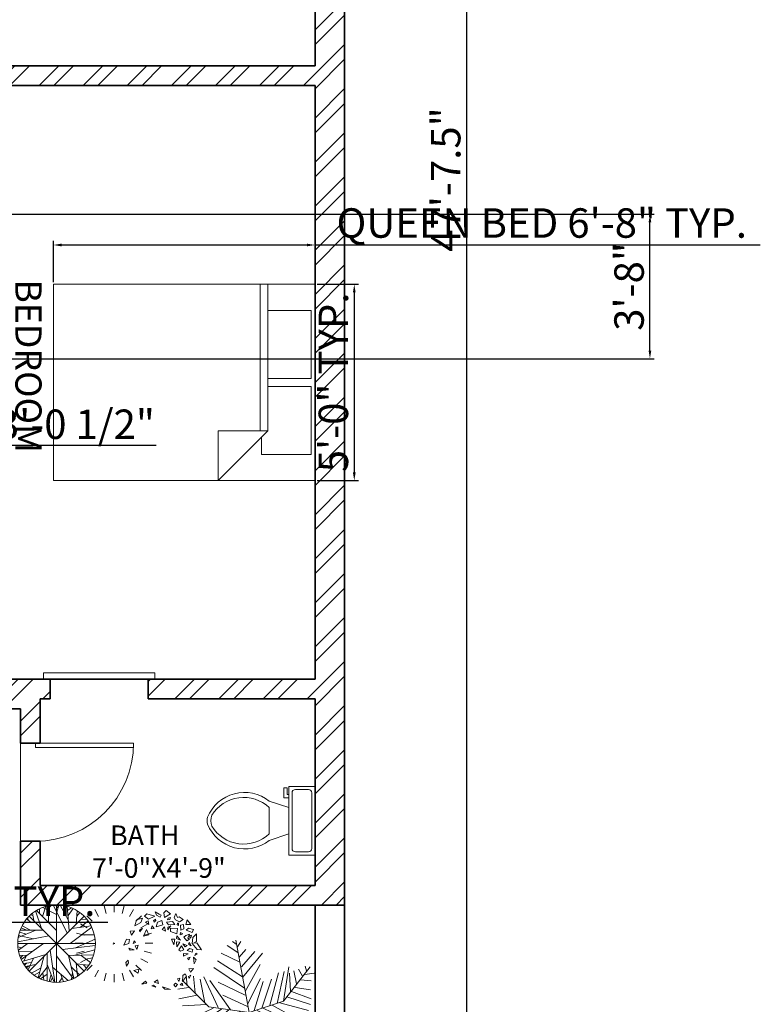
# Model space of a CAD drawing. Units: inches. Extents: x 744 to 1448, y 5126 to 6077.
# Tile 4 of 10: x 1221 to 1448, y 5284 to 5585. Entities that reach past the tile are written whole.
import ezdxf

# ---------------------------------------------------------------- set-up
doc = ezdxf.new("R2010")
doc.units = ezdxf.units.IN
for name, color, linetype, lineweight in [('A-ANNO-DIMS', 2, 'Continuous', 18), ('A-AREA-IDEN', 7, 'Continuous', 18), ('A-DOOR', 4, 'Continuous', 18), ('A-FLOR-FIXT', 9, 'Continuous', 18), ('A-FURN', 8, 'Continuous', 18), ('A-WALL', 7, 'Continuous', 35), ('A-WALL-PATT', 252, 'Continuous', 13), ('L-PLNT', 3, 'Continuous', 13)]:
    doc.layers.add(name, color=color, linetype=linetype, lineweight=lineweight)
doc.styles.get("Standard").update_dxf_attribs({"font": 'arial.ttf'})
doc.dimstyles.new('ISO-25', dxfattribs={"dimtxt": 9, "dimasz": 2.5, "dimexe": 1.25, "dimexo": 0.625, "dimtad": 1, "dimlunit": 3, "dimtxsty": 'Standard', "dimcen": 2.5, "dimadec": 0, "dimazin": 0, "dimtfac": 1, "dimtmove": 0, "dimatfit": 3, "dimfxl": 1, "dimarcsym": 0})

# ---------------------------------------------------------------- blocks, each defined once
blk = doc.blocks.new('*U3')
for p, q in [((-40, 0), (-40, 6)), ((0, 0), (0, 6))]:
    blk.add_line(p, q)
blk.add_lwpolyline([(0, 0), (0, -40), (-1.75, -40), (-1.75, 0)], close=True)
blk.add_arc((0, 0), 40, 180, 270)
blk = doc.blocks.new('*U8')
for p, q in [((9.5, -6), (9.5, -2)), ((-10, -8.5), (-8, -8.5)), ((-10, -9.5), (-10, -8.5)), ((-8, -8.5), (-8, -8)), ((-7, -8), (-7, -9.5)), ((-4, -8), (-6, -14)), ((4, -8), (6, -14)), ((-7, -9.5), (-10, -9.5)), ((4, -14), (-4, -14))]:
    blk.add_line(p, q)
blk.add_lwpolyline([(10.5, -8), (10.5, 0), (-10.5, 0), (-10.5, -8)], close=True)
for points in [[(-9.5, -2), (-9.5, -6)], [(8.5, -1), (-8.5, -1)], [(-8.5, -7), (8.5, -7)]]:
    blk.add_lwpolyline(points)
for centre, radius, start, end in [((-8.62, -1.88), 0.884, 81.8699, 188.1301), ((8.62, -1.88), 0.884, 351.8699, 98.1301), ((-8.62, -6.12), 0.884, 171.8699, 278.1301), ((8.62, -6.12), 0.884, 261.8699, 8.1301), ((3.52, -21.58), 12.17, 141.4691, 247.9714), ((4.2, -21.82), 11.33, 136.3677, 238.9468), ((-3.52, -21.58), 12.17, 292.0284, 38.5307), ((-4.2, -21.82), 11.33, 301.053, 43.6321), ((0, -27.88), 4, 245.7318, 294.2682), ((0, -29), 4, 254.8605, 285.1395)]:
    blk.add_arc(centre, radius, start, end)
blk = doc.blocks.new('*U10')
for p, q in [((-10.186, 53.64), (-13.084, 55.962)), ((0, 0), (-10.5, 57)), ((-9.099, 51.782), (-6.563, 55.962)), ((-7.288, 39.707), (-21.778, 46.673)), ((-8.737, 47.138), (-17.069, 52.711)), ((-7.65, 43.423), (-2.578, 49.46)), ((-5.839, 35.992), (4.667, 48.067)), ((-5.114, 27.632), (10.463, 46.673)), ((-5.114, 28.097), (-24.676, 40.636)), ((-3.665, 19.273), (-27.574, 35.527)), ((-2.941, 16.486), (8.652, 37.85)), ((16.259, 5.805), (23.142, 31.348)), ((22.055, 7.198), (27.489, 32.277)), ((27, 9), (48, 36)), ((27.127, 9.056), (31.112, 35.992)), ((35.096, 32.741), (37.27, 22.524)), ((38.719, 34.134), (41.979, 28.561)), ((44.153, 36.456), (45.239, 32.741)), ((-31.5, 4.5), (-52.5, 25.5)), ((-48.585, 21.131), (-49.309, 29.026)), ((-43.513, 28.561), (-42.427, 15.558)), ((-38.442, 26.239), (-34.819, 7.663)), ((-35.544, 28.097), (-24.314, 3.947)), ((-14.533, 2.09), (-30.834, 25.31)), ((-24.314, 23.917), (-2.941, 13.7)), ((-1.129, 6.734), (9.014, 26.704)), ((3.942, 1.625), (11.187, 24.381)), ((10.101, 3.483), (17.708, 26.239)), ((31.836, 30.883), (32.561, 16.486)), ((40.53, 25.775), (48.862, 24.846)), ((43.791, 29.954), (51.036, 30.883)), ((-47.498, 19.737), (-55.83, 18.344)), ((33.285, 16.486), (48.862, 10.913)), ((36.183, 19.737), (48.137, 17.88)), ((-40.615, 13.7), (-55.105, 10.913)), ((-20.691, 13.7), (-1.129, 4.876)), ((0, 0), (27, 9)), ((29.662, 12.307), (48.137, 6.269)), ((-33.37, 6.269), (-52.207, 5.34)), ((-28.299, 3.483), (-47.86, -5.805)), ((-21.416, 3.018), (-38.079, -8.128)), ((0, 0), (-31.5, 4.5)), ((-15.982, 2.09), (-30.11, -9.521)), ((0, 0), (-22.5, -19.5)), ((-6.563, 1.161), (-21.416, -8.128)), ((0, 0), (18, -22.5)), ((6.478, 1.625), (26.04, -8.592)), ((11.187, 3.483), (30.749, -5.805)), ((18.07, 5.805), (35.096, -3.483)), ((24.229, 7.663), (46.688, 1.625)), ((-6.563, -5.805), (-19.967, -9.985)), ((-4.752, -3.483), (-3.665, -14.629)), ((2.493, -3.019), (-1.491, -20.202)), ((1.769, -2.555), (24.229, -9.521)), ((5.029, -6.27), (2.131, -25.775)), ((-17.431, -15.094), (-42.789, -18.809)), ((-15.257, -12.772), (-30.11, -12.772)), ((-17.069, -15.094), (-12.721, -40.172)), ((-13.446, -11.378), (-8.737, -32.741)), ((-9.461, -8.592), (-6.201, -23.453)), ((9.014, -11.378), (3.58, -35.992)), ((7.565, -9.056), (32.198, -14.629)), ((12.274, -15.094), (36.907, -18.809)), ((-24.314, -21.596), (-42.427, -22.06)), ((-22.5, -19.5), (-37.5, -45)), ((-20.691, -18.345), (-17.793, -44.352)), ((14.085, -16.951), (6.478, -40.172)), ((18.07, -22.524), (8.289, -45.745)), ((16.259, -19.738), (36.183, -22.989)), ((18, -22.5), (27, -52.5)), ((18.433, -22.524), (40.53, -29.026)), ((-28.299, -29.026), (-42.789, -31.348)), ((-26.849, -26.24), (-40.253, -25.775)), ((-29.023, -30.884), (-27.936, -43.887)), ((-25.038, -23.918), (-22.865, -45.281)), ((20.244, -30.419), (15.897, -44.816)), ((19.157, -25.311), (38.719, -33.206)), ((-30.834, -34.135), (-42.427, -35.528)), ((-32.646, -36.921), (-31.921, -44.352)), ((22.78, -37.85), (19.519, -48.532)), ((21.331, -32.741), (39.081, -40.636)), ((22.78, -38.314), (34.372, -44.816)), ((-34.457, -39.708), (-40.978, -42.494)), ((24.591, -45.745), (23.142, -50.854)), ((24.591, -43.423), (30.749, -47.603)), ((26.764, -49.925), (28.213, -50.854))]:
    blk.add_line(p, q)
blk = doc.blocks.new('*U11')
for points in [[(1.24, 12), (0.56, 11.31), (0.76, 10.01), (2.52, 11.05)], [(-5.78, 9.75), (-7.54, 9.23), (-8.01, 7.5), (-6.26, 8.45)], [(-4.43, 11.05), (-5.18, 10.36), (-3.96, 9.49), (-2.07, 10.36)], [(-4.84, 8.63), (-3.83, 7.85), (-4.03, 8.97)], [(-1.94, 9.49), (-2.48, 8.97), (-2.27, 8.54), (-1.8, 9.06)], [(-2, 11.66), (-1.6, 10.62), (-0.52, 10.1), (-0.18, 10.62), (-0.79, 10.96)], [(0.02, 9.06), (-1.33, 8.54), (-1.73, 7.16), (0.29, 7.76)], [(1.37, 8.54), (3.13, 8.8), (3.8, 7.85), (1.91, 7.76)], [(2.59, 9.93), (1.84, 9.75), (1.64, 9.23), (2.32, 9.41)], [(4.14, 11.14), (3.6, 10.01), (4, 9.23), (5.22, 8.71), (6.3, 9.41), (5.08, 10.19), (4.61, 10.01)], [(7.45, 9.32), (7.11, 7.94), (8.52, 7.94)], [(-8.14, 6.03), (-9.36, 5.95), (-9.02, 4.73)], [(-5.78, 6.81), (-6.66, 6.21), (-6.52, 5.69)], [(-4.57, 6.38), (-5.45, 4.47), (-3.89, 4.82)], [(-2.88, 7.5), (-3.15, 6.64), (-2.27, 6.72)], [(0.76, 7.16), (0.09, 6.46), (1.1, 5.95)], [(1.71, 6.29), (1.71, 7.07), (2.65, 7.5), (2.11, 6.9)], [(2.52, 6.81), (2.52, 5.86), (4.41, 5.17), (4.61, 6.72)], [(4.61, 8.28), (4.54, 7.76), (4.95, 7.59), (4.95, 8.28)], [(6.43, 7.94), (5.49, 7.68), (5.56, 6.21), (6.5, 6.64)], [(7.85, 6.81), (7.18, 6.21), (9, 5.51), (9.33, 6.38)], [(-11.32, 1.79), (-9.83, 2.31), (-9.63, 3.44), (-10.44, 3.52)], [(-8.21, 3.09), (-8.48, 2.31), (-7.87, 2.57)], [(3.53, 1.88), (2.86, 3.52), (3.8, 3.52)], [(4.41, 4.56), (4.27, 3.7), (5.49, 3.26)], [(5.49, 5.51), (5.42, 4.82), (6.16, 5.08)], [(8.12, 4.99), (7.11, 4.65), (6.5, 4.13), (7.38, 3.09), (8.12, 3.52), (7.65, 3.87)], [(8.73, 4.73), (8.19, 4.56), (8.39, 3.87), (8.59, 4.04)], [(10.28, 5.17), (9.2, 4.04), (9, 2.31), (10.48, 0.49), (11.76, 0.41), (10.35, 2.48), (9.33, 2.4), (10.28, 2.83)], [(-8.21, 0.41), (-9.43, 0.32), (-9.83, 0.84)], [(-7, 1.79), (-7.94, 1.53), (-7.47, 0.49)], [(4.27, 2.74), (5.29, 2.66), (4.41, 1.27)], [(5.83, 1.53), (5.02, 0.41), (5.49, -0.02), (6.5, 0.41)], [(7.51, 1.71), (6.91, 1.27), (6.23, 2.14)], [(8.12, 0.75), (7.51, 0.15), (8.93, -0.28), (9.13, 0.49)], [(8.19, 2.57), (7.92, 2.05), (8.66, 1.53)], [(-10.03, -2.71), (-10.64, -3.31), (-10.44, -4.44), (-9.9, -3.49)], [(7.78, -0.8), (6.43, -1.5), (6.43, -0.72)], [(8.32, -1.75), (7.98, -2.53), (7.58, -2.1)], [(9.33, -1.75), (9.54, -3.74), (10.14, -2.53)], [(10.08, -0.63), (9.74, -1.32), (10.48, -0.89)], [(-8.28, -5.73), (-6.79, -5.3), (-7, -6.51)], [(9.33, -5.13), (8.46, -6.25), (7.98, -5.22)], [(-2.34, -9.2), (-1.26, -8.5), (-0.99, -9.54)], [(5.29, -7.98), (4.61, -8.16), (5.02, -8.94)], [(6.1, -8.94), (6.16, -7.21), (6.91, -6.69), (7.24, -7.38)], [(8.05, -8.07), (8.59, -7.12), (7.92, -7.55)], [(-4.84, -8.85), (-4.43, -9.45), (-5.99, -9.8)], [(-2.54, -10.06), (-3.02, -10.23), (-1.8, -10.67)], [(0.22, -10.58), (0.83, -11.27), (2.59, -11.36)], [(4.07, -9.45), (3.53, -9.97), (4.07, -10.58), (4.61, -9.89)], [(6.03, -9.45), (5.42, -9.97), (6.16, -10.15)]]:
    blk.add_lwpolyline(points, close=True)
blk = doc.blocks.new('*U12')
for p, q in [((-25.024, 42.079), (-31.077, 52.563)), ((-13.435, 46.72), (-16.606, 58.557)), ((-1.077, 60.601), (-1.077, 48.601)), ((11.28, 46.72), (14.452, 58.557)), ((22.87, 42.079), (28.923, 52.563)), ((-42.564, 24.554), (-53.039, 30.601)), ((-34.93, 34.454), (-43.503, 43.028)), ((32.776, 34.454), (41.349, 43.028)), ((40.409, 24.554), (50.884, 30.601)), ((-47.5, 13.04), (-59.033, 16.131)), ((45.346, 13.04), (56.878, 16.131)), ((-61.077, 0.601), (-49.077, 0.601)), ((58.923, 0.601), (46.923, 0.601)), ((-47.5, -11.837), (-59.033, -14.928)), ((45.346, -11.837), (56.878, -14.928)), ((-42.564, -23.351), (-53.039, -29.399)), ((40.409, -23.351), (50.884, -29.399)), ((-34.93, -33.251), (-43.503, -41.825)), ((-25.024, -40.876), (-31.077, -51.36)), ((-13.435, -45.517), (-16.606, -57.354)), ((11.28, -45.517), (14.452, -57.354)), ((22.87, -40.876), (28.923, -51.36)), ((32.776, -33.251), (41.349, -41.825)), ((-1.077, -59.399), (-1.077, -47.399))]:
    blk.add_line(p, q)
blk.add_lwpolyline([(-1.908, 0.978), (-2.67, -0.978), (0, 0)], close=True)
blk = doc.blocks.new('*U13')
for p, q in [((-37.0107, 47.0408), (-35.25, 35.5298)), ((-32.6092, 50.4264), (-23.2782, 23.5674)), ((-31.2008, 51.1035), (-0.2149, 20.1818)), ((-26.4472, 46.5894), (-26.2712, 53.8116)), ((-22.0458, 42.0753), (-16.5881, 57.6486)), ((-21.1656, 55.8436), (-0.0388, 45.0094)), ((-12.5388, 54.9406), (-7.9613, 59.4546)), ((-12.3627, 32.1443), (-12.5388, 58.7776)), ((-5.3205, 59.6806), (16.5105, 16.7963)), ((2.426, 54.9406), (-1.4472, 59.9056)), ((0, 59.9996), (0, -60)), ((0.4894, 48.6208), (3.6584, 59.6806)), ((18.2711, 35.5298), (5.419, 59.6806)), ((9.8203, 51.5549), (12.8133, 58.5516)), ((19.6795, 19.5047), (16.3344, 57.6486)), ((17.0387, 51.1035), (23.2006, 55.1666)), ((17.7429, 43.6552), (25.4894, 54.2636)), ((31.6513, 50.8778), (30.2429, 30.5643)), ((31.1232, 42.5267), (35.8767, 48.1693)), ((-49.8627, 32.8214), (-32.7853, 32.8214)), ((-45.8134, 38.2383), (-40.5318, 33.0471)), ((-43.8768, 36.4326), (-44.405, 40.2696)), ((42, 42), (-42, -42)), ((42, -42), (-42, 42)), ((-40.1797, 44.558), (-36.4825, 43.2038)), ((36.2288, 25.1474), (48.9049, 35.0784)), ((37.1091, 37.1098), (46.6161, 37.5612)), ((-32.2571, 20.6333), (-59.1937, 9.348)), ((-57.081, 17.9248), (-47.0458, 14.7649)), ((-56.0247, 20.859), (-20.8134, 20.859)), ((-54.7923, 24.4702), (-47.75, 21.0847)), ((-53.2078, 27.4044), (-40.1797, 20.859)), ((54.3626, 25.3731), (20.9119, 0.3198)), ((23.3767, 23.3417), (53.3063, 27.4044)), ((-59.7219, 2.8025), (-12.0106, 12.0565)), ((-58.6656, 12.7336), (-35.9543, 7.5424)), ((-54.6162, -24.7335), (-20.2853, 0.0941)), ((29.3626, -6.6771), (59.4682, 7.091)), ((38.5175, 13.4107), (58.2359, 13.6364)), ((-60, 0), (60, 0)), ((-59.7219, -4.8714), (-54.2641, -6.6771)), ((-45.2853, -0.1316), (-59.0177, -10.0627)), ((-58.4895, -12.3197), (-36.4825, -11.6426)), ((-14.8275, -15.0282), (-14.6515, -57.6865)), ((-10.074, -10.0627), (-2.5036, -59.7178)), ((9.2922, -9.1598), (59.6443, -2.8401)), ((26.3697, -18.4138), (58.9401, -9.8369)), ((-57.081, -18.4138), (-45.2853, -17.9624)), ((-52.6797, -18.188), (-55.4966, -22.0251)), ((-53.2078, -27.442), (-16.7641, -16.6081)), ((-38.9472, -29.0219), (-51.4472, -30.6018)), ((-47.2219, -19.3166), (-50.2148, -26.3135)), ((-46.5177, -30.1504), (-49.5106, -33.536)), ((-35.9543, -22.4765), (-44.0529, -40.5329)), ((-19.9331, -20.2194), (-28.5599, -52.721)), ((-0.0388, -19.0909), (25.8415, -53.8495)), ((18.6232, -18.6394), (26.7218, -53.3981)), ((18.7992, -18.6394), (57.3556, -17.2853)), ((30.419, -30.1504), (32.3556, -50.0125)), ((38.1654, -18.188), (52.426, -29.0219)), ((45.9119, -24.0564), (55.595, -22.2508)), ((-32.4331, -32.4075), (-48.1021, -35.5674)), ((-43.7008, -34.6645), (-46.6937, -37.373)), ((-24.6867, -37.8244), (-38.7712, -45.7241)), ((-26.2712, -43.9185), (-34.7219, -48.6583)), ((-14.6515, -36.2445), (-27.6797, -52.9467)), ((-21.5177, -45.4984), (-19.9331, -56.1065)), ((-14.6515, -32.1818), (-3.912, -59.4922)), ((-6.2008, -36.2445), (17.919, -57.0094)), ((22.8485, -36.4702), (35.3485, -48.4326)), ((24.7852, -44.8213), (23.0246, -54.978)), ((31.4753, -31.279), (49.6091, -33.3103)), ((41.5105, -32.6332), (46.088, -38.0501)), ((-14.6515, -47.3041), (-25.0388, -54.3009)), ((-8.4895, -47.5298), (-11.4825, -58.5893)), ((-6.3768, -52.721), (-9.3698, -58.815)), ((8.4119, -53.1724), (3.8344, -59.4922)), ((5.9471, -46.6269), (10.5246, -58.5893))]:
    blk.add_line(p, q)
blk.add_circle((0, 0), 60)
blk = doc.blocks.new('Bed - Queen')
for p, q in [((0, -80.00003), (0, 0)), ((0, 0), (59.99999, 0)), ((59.99999, 0), (59.99999, -80.00003)), ((7.99999, -1.2), (28.79998, -1.2)), ((7.99999, -14.4), (7.99999, -1.2)), ((28.79998, -1.2), (28.79998, -14.4)), ((31.19999, -1.2), (51.99999, -1.2)), ((31.19999, -14.4), (31.19999, -1.2)), ((51.99999, -1.2), (51.99999, -16.4)), ((0, -14.4), (44.8, -14.4)), ((59.99999, -29.6), (44.8, -14.4)), ((44.8, -14.4), (44.8, -29.6)), ((44.8, -16.8), (0, -16.8)), ((51.99999, -16.4), (46.79936, -16.4)), ((44.8, -29.6), (59.99999, -29.6)), ((59.99999, -80.00003), (0, -80.00003))]:
    blk.add_line(p, q)
blk = doc.blocks.new('*D23')
at = {"layer": 'A-ANNO-DIMS', "color": 0, "lineweight": -2, "transparency": 16777216}
for p, q in [((1321.31, 5821.82), (1359.26, 5821.82)), ((1358.01, 5819.32), (1358.01, 5252.82)), ((1321.31, 5250.32), (1359.26, 5250.32))]:
    blk.add_line(p, q, dxfattribs=at)
at = {"layer": 'A-ANNO-DIMS', "color": 0, "transparency": 16777216}
for points in [[(1357.59, 5819.32), (1358.42, 5819.32), (1358.01, 5821.82)], [(1357.59, 5252.82), (1358.42, 5252.82), (1358.01, 5250.32)]]:
    blk.add_solid(points, dxfattribs=at)
at = {"layer": 'Defpoints', "color": 0, "transparency": 16777216}
for p in [(1320.68, 5821.82), (1320.68, 5250.32), (1358.01, 5250.32)]:
    blk.add_point(p, dxfattribs=at)
at = {"layer": 'A-ANNO-DIMS', "color": 0, "transparency": 16777216, "insert": (1352.81, 5536.07), "char_height": 9, "attachment_point": 5, "rotation": 90}
blk.add_mtext('47\'-7.5"', dxfattribs=at)
blk = doc.blocks.new('*D31')
at = {"layer": 'A-ANNO-DIMS', "color": 0, "lineweight": -2, "transparency": 16777216}
for p, q in [((1231.68, 5504.69), (1231.68, 5517.32)), ((1311.68, 5504.69), (1311.68, 5517.32)), ((1234.18, 5516.07), (1309.18, 5516.07)), ((1311.68, 5516.07), (1447.83, 5516.07))]:
    blk.add_line(p, q, dxfattribs=at)
at = {"layer": 'A-ANNO-DIMS', "color": 0, "transparency": 16777216}
for points in [[(1234.18, 5516.48), (1234.18, 5515.65), (1231.68, 5516.07)], [(1309.18, 5516.48), (1309.18, 5515.65), (1311.68, 5516.07)]]:
    blk.add_solid(points, dxfattribs=at)
at = {"layer": 'Defpoints', "color": 0, "transparency": 16777216}
for p in [(1311.68, 5516.07), (1231.68, 5504.07), (1311.68, 5504.07)]:
    blk.add_point(p, dxfattribs=at)
at = {"layer": 'A-ANNO-DIMS', "color": 0, "transparency": 16777216, "insert": (1381, 5521.62), "char_height": 9, "attachment_point": 5}
blk.add_mtext('QUEEN BED 6\'-8" TYP.', dxfattribs=at)
blk = doc.blocks.new('*D32')
at = {"layer": 'A-ANNO-DIMS', "color": 0, "lineweight": -2, "transparency": 16777216}
for p, q in [((1312.31, 5504.07), (1324.93, 5504.07)), ((1323.68, 5501.57), (1323.68, 5446.57)), ((1312.31, 5444.07), (1324.93, 5444.07))]:
    blk.add_line(p, q, dxfattribs=at)
at = {"layer": 'A-ANNO-DIMS', "color": 0, "transparency": 16777216}
for points in [[(1323.27, 5501.57), (1324.1, 5501.57), (1323.68, 5504.07)], [(1323.27, 5446.57), (1324.1, 5446.57), (1323.68, 5444.07)]]:
    blk.add_solid(points, dxfattribs=at)
at = {"layer": 'Defpoints', "color": 0, "transparency": 16777216}
for p in [(1311.68, 5504.07), (1311.68, 5444.07), (1323.68, 5444.07)]:
    blk.add_point(p, dxfattribs=at)
at = {"layer": 'A-ANNO-DIMS', "color": 0, "transparency": 16777216, "insert": (1318.46, 5474.07), "char_height": 9, "attachment_point": 5, "rotation": 90}
blk.add_mtext('5\'-0" TYP.', dxfattribs=at)
blk = doc.blocks.new('*D37')
at = {"layer": 'A-ANNO-DIMS', "color": 0, "lineweight": -2, "transparency": 16777216}
for p, q in [((1063.79, 5316.69), (1063.79, 5307.82)), ((1118.79, 5316.69), (1118.79, 5307.82)), ((1066.29, 5309.07), (1116.29, 5309.07)), ((1118.79, 5309.07), (1248.3, 5309.07))]:
    blk.add_line(p, q, dxfattribs=at)
at = {"layer": 'A-ANNO-DIMS', "color": 0, "transparency": 16777216}
for points in [[(1066.29, 5309.48), (1066.29, 5308.65), (1063.79, 5309.07)], [(1116.29, 5309.48), (1116.29, 5308.65), (1118.79, 5309.07)]]:
    blk.add_solid(points, dxfattribs=at)
at = {"layer": 'Defpoints', "color": 0, "transparency": 16777216}
for p in [(1063.79, 5317.32), (1118.79, 5317.32), (1118.79, 5309.07)]:
    blk.add_point(p, dxfattribs=at)
at = {"layer": 'A-ANNO-DIMS', "color": 0, "transparency": 16777216, "insert": (1184.8, 5314.35), "char_height": 9, "attachment_point": 5}
blk.add_mtext('WINDOW A 4\'-7" TYP.', dxfattribs=at)
blk = doc.blocks.new('*D61')
at = {"layer": 'A-ANNO-DIMS', "color": 0, "lineweight": -2, "transparency": 16777216}
for p, q in [((905.31, 5525.47), (1415.33, 5525.47)), ((1414.08, 5483.82), (1414.08, 5522.97)), ((905.31, 5481.32), (1415.33, 5481.32))]:
    blk.add_line(p, q, dxfattribs=at)
at = {"layer": 'A-ANNO-DIMS', "color": 0, "transparency": 16777216}
for points in [[(1413.67, 5522.97), (1414.5, 5522.97), (1414.08, 5525.47)], [(1413.67, 5483.82), (1414.5, 5483.82), (1414.08, 5481.32)]]:
    blk.add_solid(points, dxfattribs=at)
at = {"layer": 'Defpoints', "color": 0, "transparency": 16777216}
for p in [(904.68, 5525.47), (1414.08, 5525.47), (904.68, 5481.32)]:
    blk.add_point(p, dxfattribs=at)
at = {"layer": 'A-ANNO-DIMS', "color": 0, "transparency": 16777216, "insert": (1408.86, 5503.39), "char_height": 9, "attachment_point": 5, "rotation": 90}
blk.add_mtext('3\'-8"', dxfattribs=at)
blk = doc.blocks.new('*D65')
at = {"layer": 'A-ANNO-DIMS', "color": 0, "lineweight": -2, "transparency": 16777216}
for p, q in [((1141.21, 5454.83), (1177.84, 5454.83)), ((1263.08, 5454.83), (1180.34, 5454.83))]:
    blk.add_line(p, q, dxfattribs=at)
at = {"layer": 'A-ANNO-DIMS', "color": 0, "transparency": 16777216}
blk.add_solid([(1180.34, 5455.25), (1180.34, 5454.41), (1177.84, 5454.83)], dxfattribs=at)
at = {"layer": 'Defpoints', "color": 0, "transparency": 16777216}
for p in [(1141.21, 5454.83), (1177.84, 5454.83)]:
    blk.add_point(p, dxfattribs=at)
at = {"layer": 'A-ANNO-DIMS', "color": 0, "transparency": 16777216, "insert": (1222.96, 5460.11), "char_height": 9, "attachment_point": 5, "rotation": 0.0006}
blk.add_mtext('12X R3\'-0 1/2"', dxfattribs=at)

msp = doc.modelspace()

# ---------------------------------------------------------------- hatches: boundary and pattern name
at = {"layer": 'A-WALL-PATT'}
h = msp.add_hatch(dxfattribs=at)
h.set_pattern_fill('ANSI32', color=256)
h.paths.add_polyline_path([(813.684, 5750.816), (876.684, 5750.816), (876.684, 5756.816), (813.684, 5756.816), (813.684, 5812.816), (909.684, 5812.816), (909.684, 5795.316), (915.684, 5795.316), (915.684, 5812.816), (1209.684, 5812.816), (1209.684, 5795.316), (1215.684, 5795.316), (1215.684, 5812.816), (1311.684, 5812.816), (1311.684, 5756.816), (1248.684, 5756.816), (1248.684, 5750.816), (1311.684, 5750.816), (1311.684, 5570.816), (1179.044, 5570.816), (1179.044, 5564.816), (1311.684, 5564.816), (1311.684, 5383.316), (1260.684, 5383.316), (1260.684, 5377.316), (1311.684, 5377.316), (1311.684, 5320.316), (1227.684, 5320.316), (1227.684, 5333.816), (1221.684, 5333.816), (1221.684, 5314.316), (1320.684, 5314.316), (1320.684, 5821.816), (804.684, 5821.816), (804.684, 5472.316), (926.184, 5472.316), (926.184, 5481.316), (813.684, 5481.316), (813.684, 5581.616), (946.284, 5581.616), (946.284, 5587.616), (813.684, 5587.616)])
h.paths.add_polyline_path([(1155.684, 5525.816), (1149.684, 5525.816), (1149.684, 5481.316), (1025.184, 5481.316), (1025.184, 5475.316), (1146.684, 5475.316), (1146.684, 5323.316), (1118.788, 5323.316), (1118.788, 5314.316), (1146.684, 5314.316), (1155.684, 5314.316), (1155.684, 5374.316), (1170.35, 5374.316), (1170.35, 5383.316), (1155.684, 5383.316)], flags=17)
h.paths.add_polyline_path([(1230.684, 5383.316), (1213.35, 5383.316), (1213.35, 5374.316), (1221.684, 5374.316), (1221.684, 5363.816), (1226.184, 5363.816), (1227.684, 5363.816), (1227.684, 5377.316), (1230.684, 5377.316)], flags=17)
h.paths.add_polyline_path([(1185.684, 5671.816), (1155.684, 5671.816), (1155.684, 5750.816), (1161.575, 5750.816), (1161.575, 5756.816), (1157.542, 5756.816), (1157.847, 5756.715), (1155.79, 5756.816), (1149.684, 5756.816), (1149.684, 5750.816), (1149.684, 5671.816), (1121.684, 5671.816), (1121.684, 5665.816), (1179.684, 5665.816), (1179.684, 5609.816), (1185.684, 5609.816)], flags=17)
h.paths.add_polyline_path([(1003.684, 5671.816), (975.684, 5671.816), (975.684, 5750.816), (975.684, 5756.816), (965.205, 5756.816), (965.205, 5750.816), (969.684, 5750.816), (969.684, 5671.816), (939.684, 5671.816), (939.684, 5626.616), (945.684, 5626.616), (945.684, 5665.816), (1003.684, 5665.816)], flags=17)
h.paths.add_polyline_path([(915.684, 5774.316), (909.684, 5774.316), (909.684, 5756.816), (906.684, 5756.816), (906.684, 5752.316), (906.684, 5750.816), (922.205, 5750.816), (922.205, 5756.816), (915.684, 5756.816)], flags=17)
h.paths.add_polyline_path([(1215.684, 5774.316), (1209.684, 5774.316), (1209.684, 5756.816), (1204.575, 5756.816), (1204.575, 5750.816), (1218.684, 5750.816), (1218.684, 5756.816), (1215.684, 5756.816)], flags=17)
h.paths.add_polyline_path([(1063.788, 5323.316), (1025.184, 5323.316), (1025.184, 5314.316), (1063.788, 5314.316)])
h.paths.add_polyline_path([(986.184, 5475.316), (989.184, 5475.316), (989.184, 5481.316), (974.184, 5481.316), (974.184, 5475.916), (974.184, 5472.316), (977.184, 5472.316), (977.184, 5314.316), (989.184, 5314.316), (989.184, 5319.716), (989.184, 5323.316), (986.184, 5323.316)])

# ---------------------------------------------------------------- linework, layer by layer
at = {"layer": 'A-DOOR'}
for p, q in [((1228.684, 5385.316), (1262.684, 5385.316)), ((1228.684, 5383.316), (1228.684, 5385.316)), ((1262.684, 5383.316), (1262.684, 5385.316)), ((1221.684, 5333.816), (1221.684, 5363.816))]:
    msp.add_line(p, q, dxfattribs=at)
at = {"layer": 'A-WALL'}
for p, q in [((1320.684, 5250.316), (1320.684, 5821.816)), ((1311.684, 5570.816), (1311.684, 5750.816)), ((1179.044, 5570.816), (1311.684, 5570.816)), ((1155.684, 5564.816), (1311.684, 5564.816)), ((1311.684, 5383.316), (1311.684, 5564.816)), ((1155.684, 5383.316), (1311.684, 5383.316)), ((1230.684, 5377.316), (1230.684, 5383.316)), ((1260.684, 5377.316), (1260.684, 5383.316)), ((1227.684, 5377.316), (1230.684, 5377.316)), ((1227.684, 5363.816), (1227.684, 5377.316)), ((1260.684, 5377.316), (1311.684, 5377.316)), ((1311.684, 5320.316), (1311.684, 5377.316)), ((1155.684, 5374.316), (1221.684, 5374.316)), ((1221.684, 5363.816), (1221.684, 5374.316)), ((1227.684, 5363.816), (1221.684, 5363.816)), ((1221.684, 5314.316), (1221.684, 5333.816)), ((1227.684, 5333.816), (1221.684, 5333.816)), ((1227.684, 5320.316), (1227.684, 5333.816)), ((1227.684, 5320.316), (1311.684, 5320.316)), ((1221.684, 5314.316), (1320.684, 5314.316)), ((1311.684, 5256.316), (1311.684, 5314.316))]:
    msp.add_line(p, q, dxfattribs=at)

# ---------------------------------------------------------------- block references
at = {"layer": 'A-DOOR', "xscale": 0.75, "yscale": 0.75, "zscale": 0.75, "rotation": 89.99999999999969}
msp.add_blockref('*U3', (1226.184, 5363.816), dxfattribs=at)
at = {"layer": 'A-FLOR-FIXT', "rotation": 270}
msp.add_blockref('*U8', (1311.684, 5340.106), dxfattribs=at)
at = {"layer": 'A-FURN', "rotation": 270}
msp.add_blockref('Bed - Queen', (1311.684, 5504.066), dxfattribs=at)
at = {"layer": 'L-PLNT'}
for name, p, xscale, yscale, zscale in [('*U13', (1232.666, 5302.543), 0.1976487053468327, 0.1976487053468327, 0.1976487053468327), ('*U12', (1250.466, 5302.543), 0.1976487053468327, 0.1976487053468327, 0.1976487053468327), ('*U11', (1264.871, 5300.233), 1.032484677762128, 1.032484677762128, 1.032484677762128), ('*U10', (1291.509, 5281.439), 0.3894195221065574, 0.3894195221065574, 0.3894195221065574)]:
    msp.add_blockref(name, p, dxfattribs=dict(at, xscale=xscale, yscale=yscale, zscale=zscale))

# ---------------------------------------------------------------- texts
at = {"layer": 'A-AREA-IDEN', "insert": (1228.074, 5510.459), "char_height": 8, "attachment_point": 1, "rotation": 270}
msp.add_mtext_dynamic_manual_height_columns('  BEDROOM\\P13\'-0"X15\'-1.5"', width=73.67045, gutter_width=12.5, heights=[0], dxfattribs=at)
at = {"layer": 'A-AREA-IDEN', "insert": (1243.514, 5338.655), "char_height": 6, "attachment_point": 1}
msp.add_mtext_dynamic_manual_height_columns('   BATH\\P7\'-0"X4\'-9"', width=39.96322, gutter_width=12.5, heights=[0], dxfattribs=at)

# ---------------------------------------------------------------- dimensions: what is measured, and where the dimension line sits
at = {"layer": 'A-ANNO-DIMS'}
for base, p1, p2, override, picture, middle in [((1358.008, 5250.316), (1320.684, 5821.816), (1320.684, 5250.316), {"dimclrd": 0, "dimclre": 0, "dimclrt": 0}, '*D23', (1352.806, 5536.066)), ((1414.084316, 5525.465662), (904.684316, 5481.315662), (904.684316, 5525.465662), {"dimdec": 1, "dimlfac": 1, "dimrnd": 0, "dimzin": 1, "dimdsep": 46, "dimlunit": 4, "dimfrac": 2}, '*D61', (1408.861089533, 5503.390662))]:
    dim = msp.add_linear_dim(base=base, p1=p1, p2=p2, angle=90, dimstyle='ISO-25', override=override, dxfattribs=at)
    dim.commit()
    dim.dimension.update_dxf_attribs({"geometry": picture, "text_midpoint": middle})
for base, p1, p2, text, picture, middle in [((1311.684, 5516.066), (1231.684, 5504.066), (1311.684, 5504.066), 'QUEEN BED <> TYP.', '*D31', (1381.005, 5521.62)), ((1118.788, 5309.066), (1063.788, 5317.316), (1118.788, 5317.316), 'WINDOW A <> TYP.', '*D37', (1184.796, 5314.347))]:
    dim = msp.add_linear_dim(base=base, p1=p1, p2=p2, text=text, dimstyle='ISO-25', override={"dimdec": 1, "dimlfac": 1, "dimrnd": 0, "dimzin": 1, "dimdsep": 46, "dimlunit": 4, "dimfrac": 2}, dxfattribs=at)
    dim.commit()
    dim.dimension.update_dxf_attribs({"geometry": picture, "text_midpoint": middle})
dim = msp.add_linear_dim(base=(1323.684, 5444.066), p1=(1311.684, 5504.066), p2=(1311.684, 5444.066), angle=270, text='<> TYP.', dimstyle='ISO-25', override={"dimdec": 1, "dimlfac": 1, "dimrnd": 0, "dimzin": 1, "dimdsep": 46, "dimlunit": 4, "dimfrac": 2}, dxfattribs=at)
dim.commit()
dim.dimension.update_dxf_attribs({"geometry": '*D32', "text_midpoint": (1318.464, 5474.066)})
dim = msp.add_radius_dim(center=(1141.211, 5454.831), mpoint=(1177.836, 5454.831), text='12X <>', dimstyle='ISO-25', override={"dimdec": 1, "dimlfac": 1, "dimrnd": 0, "dimzin": 1, "dimdsep": 46, "dimlunit": 4, "dimfrac": 2}, dxfattribs=at)
dim.commit()
dim.dimension.update_dxf_attribs({"geometry": '*D65', "text_midpoint": (1222.958, 5460.113)})

doc.saveas('drawing.dxf')
